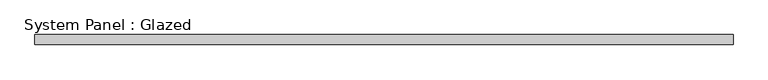
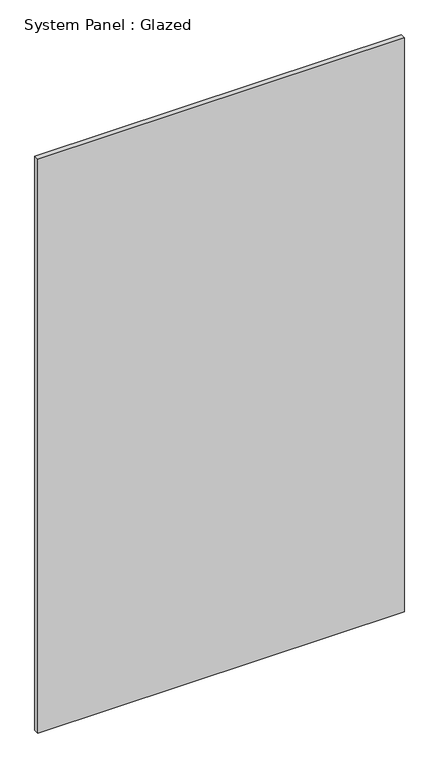
"""IFC4 building model written with IfcOpenShell, lengths in millimetres: plate geometry, System Panel : Glazed."""

from ifc_helpers import new_model, si_unit, origin, origin_with_axes, place, context, project, spatial, polyline, outline, extrude, source, transform, mapped, element, save


def system_panel_glazed_5d99744d(model_context):
    return source(origin(), model_context, "Body", "SweptSolid", [
        extrude(outline(polyline([(882.65, 19.05), (-882.65, 19.05), (-882.65, 44.45), (882.65, 44.45), (882.65, 19.05)])), origin_with_axes(), (0.0, 0.0, 1.0), 2921.0),
    ])


if __name__ == "__main__":
    model = new_model("IFC4")
    model_context = context("Model", 3, world=origin())
    ifc_project = project(units=[si_unit("LENGTHUNIT", "METRE", prefix="MILLI")], contexts=[model_context])
    site = spatial("IfcSite", under=ifc_project)
    building = spatial("IfcBuilding", under=site)
    placement = place(None, origin())
    system_panel_glazed_shape = system_panel_glazed_5d99744d(model_context)
    element("IfcPlate", 1, ObjectType="System Panel : Glazed", at=placement, inside=building, context=model_context, shape_type="MappedRepresentation", body=[
        mapped(system_panel_glazed_shape, transform((0.0, 0.0, 0.0), x_axis=(1.0, 0.0, 0.0), y_axis=(0.0, 1.0, 0.0), z_axis=(0.0, 0.0, 1.0))),
    ])
    save(model, "model.ifc")

# Revit data of these elements
# Type "System Panel : Glazed"
#   Construction Type Id = "GSP4R"
#   Analytic Construction = "1/8 in Pilkington single glazing"
#   Visual Light Transmittance = 0.9
#   Solar Heat Gain Coefficient = 0.86
#   Heat Transfer Coefficient (U) = 1.18115 BTU/(h·ft²·°F)
# Element 1 (IfcPlate, "System Panel : Glazed")
#   Materials on its faces: "Glass"
# Materials
#   "Glass": class "Glass", colour RGB 0 128 192, transparency 0.75, Description = "Soda Lime Glass", Cost = 0
